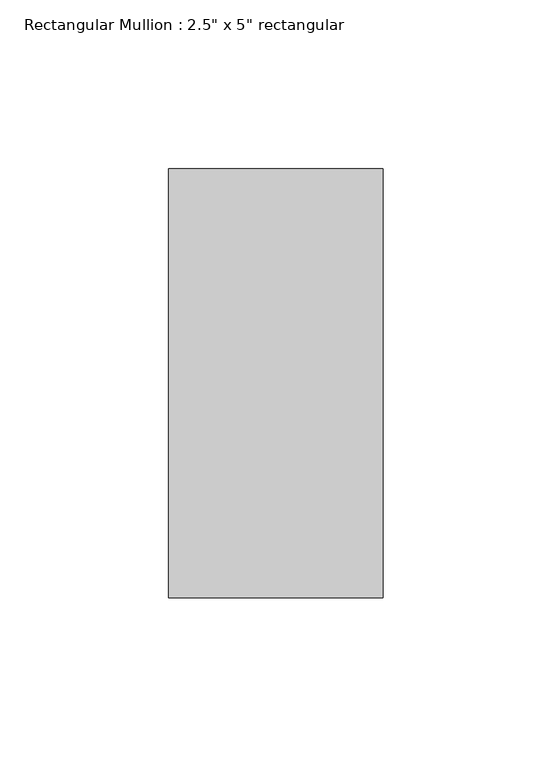
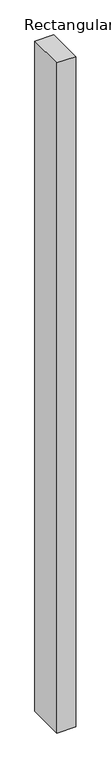
"""IFC4 building model written with IfcOpenShell, lengths in millimetres: member geometry."""

from ifc_helpers import new_model, si_unit, frame, origin, place, context, project, spatial, polyline, outline, extrude, source, transform, mapped, element, save


def member_15dc5290(model_context):
    return source(origin(), model_context, "Body", "SweptSolid", [
        extrude(outline(polyline([(0.0, 63.5), (0.0, -63.5), (-63.5, -63.5), (-63.5, 63.5), (0.0, 63.5)])), frame((0.0, 0.0, -2370.2380434), z_axis=(0.0, 0.0, 1.0), x_axis=(1.0, 0.0, 0.0)), (0.0, 0.0, 1.0), 2370.2380434),
    ])


if __name__ == "__main__":
    model = new_model("IFC4")
    model_context = context("Model", 3, world=origin())
    ifc_project = project(units=[si_unit("LENGTHUNIT", "METRE", prefix="MILLI")], contexts=[model_context])
    site = spatial("IfcSite", under=ifc_project)
    building = spatial("IfcBuilding", under=site)
    placement = place(None, origin())
    member_shape = member_15dc5290(model_context)
    element("IfcMember", 1, ObjectType="Rectangular Mullion : 2.5\" x 5\" rectangular", at=placement, inside=building, context=model_context, shape_type="MappedRepresentation", body=[
        mapped(member_shape, transform((0.0, 0.0, 0.0), x_axis=(1.0, 0.0, 0.0), y_axis=(0.0, 1.0, 0.0), z_axis=(0.0, 0.0, 1.0))),
    ])
    save(model, "model.ifc")

# Revit data of these elements
# Type "Rectangular Mullion : 2.5\" x 5\" rectangular"
#   built-in parameter 1007304 = 0.416667 (stored number, unit not read)
#   built-in parameter 1007301 = 0.104167 (stored number, unit not read)
#   built-in parameter 1007300 = 0.104167 (stored number, unit not read)
# Element 1 (IfcMember, "Rectangular Mullion : 2.5\" x 5\" rectangular")
#   Materials on its faces: "Aluminum"
# Materials
#   "Aluminum": class "Metal", colour RGB 247 247 247, transparency 0, Description = "Aluminum 6061", Cost = 0
